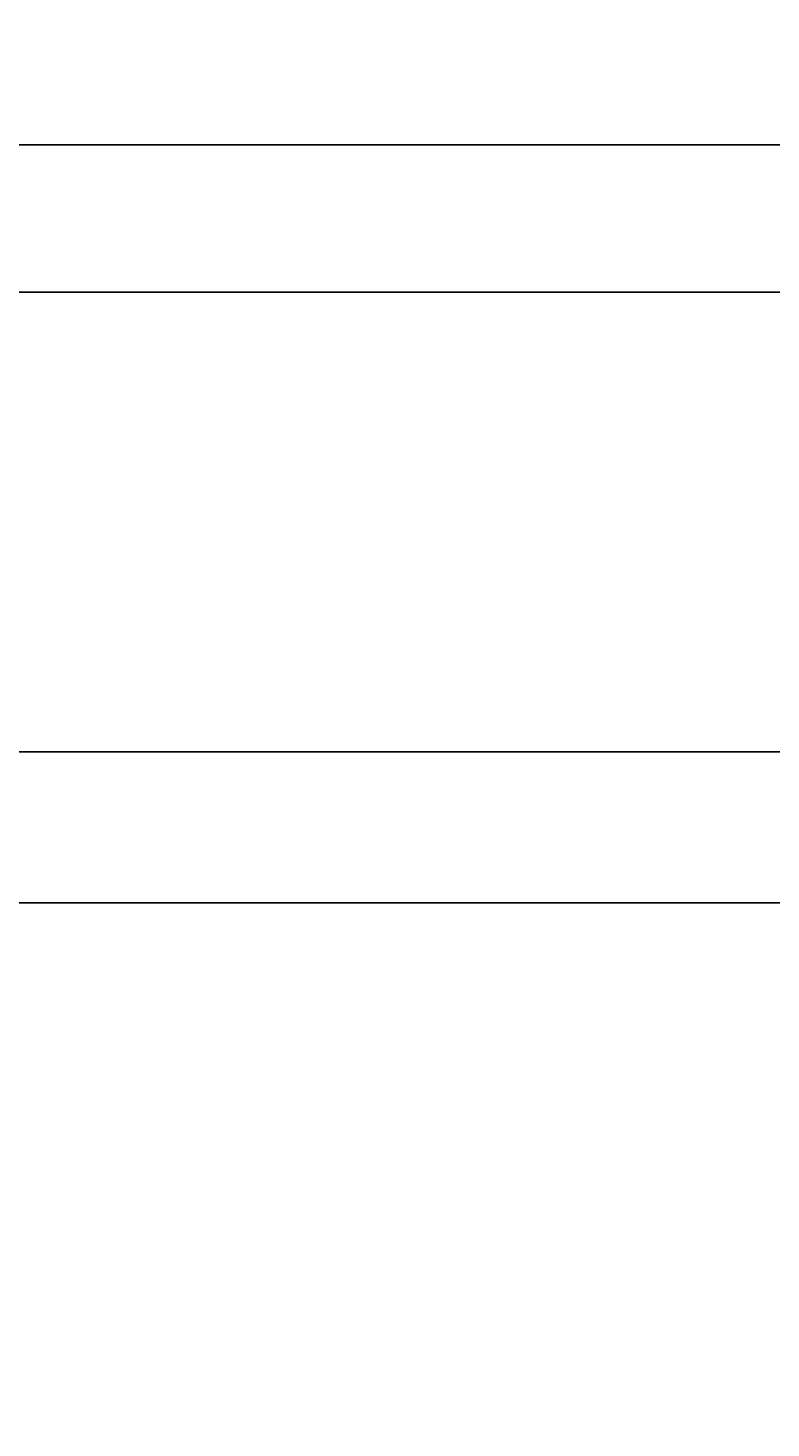
# Model space of a CAD drawing. Units: inches. Extents: x 35362 to 73946, y 43607 to 67532.
# Tile 73 of 134: x 49302 to 49711, y 46919 to 47689. Entities that reach past the tile are written whole.
import ezdxf

# ---------------------------------------------------------------- set-up
doc = ezdxf.new("R2010")
doc.units = ezdxf.units.IN
doc.header["$MEASUREMENT"] = 0
doc.layers.add('A-ANNO-DIMS', color=2, linetype='Continuous', lineweight=18)
doc.styles.get("Standard").update_dxf_attribs({"font": 'arial.ttf'})
doc.dimstyles.get("Standard").update_dxf_attribs({"dimtxt": 0.18, "dimasz": 0.18, "dimexe": 0.18, "dimexo": 0.0625, "dimgap": 0.09, "dimtad": 0, "dimtih": 1, "dimtoh": 1, "dimdec": 4, "dimzin": 0, "dimdsep": 46, "dimtxsty": 'Standard', "dimcen": 0.09, "dimadec": 0, "dimazin": 0, "dimtfac": 1, "dimtdec": 4, "dimtofl": 0, "dimtmove": 0, "dimatfit": 3, "dimfxl": 1, "dimtolj": 1, "dimtzin": 0, "dimarcsym": 0})

# ---------------------------------------------------------------- blocks, each defined once
blk = doc.blocks.new('*D11')
at = {"layer": 'A-ANNO-DIMS', "color": 0, "lineweight": -2, "transparency": 16777216}
for p, q in [((47978.66, 56028.77), (47978.66, 43606.68)), ((53109.76, 56028.77), (53109.76, 43606.68)), ((47978.84, 43606.86), (50543.87, 43606.86)), ((53109.58, 43606.86), (50544.55, 43606.86))]:
    blk.add_line(p, q, dxfattribs=at)
at = {"layer": 'A-ANNO-DIMS', "color": 0, "transparency": 16777216}
for points in [[(47978.84, 43606.89), (47978.84, 43606.83), (47978.66, 43606.86)], [(53109.58, 43606.89), (53109.58, 43606.83), (53109.76, 43606.86)]]:
    blk.add_solid(points, dxfattribs=at)
at = {"layer": 'Defpoints', "color": 0, "transparency": 16777216}
for p in [(47978.66, 56028.84), (53109.76, 56028.84), (53109.76, 43606.86)]:
    blk.add_point(p, dxfattribs=at)
at = {"layer": 'A-ANNO-DIMS', "color": 0, "transparency": 16777216, "insert": (50544.21, 43606.86), "char_height": 0.18, "attachment_point": 5}
blk.add_mtext('\\A1;5131', dxfattribs=at)
blk = doc.blocks.new('*D13')
at = {"layer": 'A-ANNO-DIMS', "color": 0, "lineweight": -2, "transparency": 16777216}
for p, q in [((48373.49, 51694.02), (48373.49, 43606.68)), ((51029.04, 51694.02), (51029.04, 43606.68)), ((48373.67, 43606.86), (49700.8, 43606.86)), ((51028.86, 43606.86), (49701.73, 43606.86))]:
    blk.add_line(p, q, dxfattribs=at)
at = {"layer": 'A-ANNO-DIMS', "color": 0, "transparency": 16777216}
for points in [[(48373.67, 43606.89), (48373.67, 43606.83), (48373.49, 43606.86)], [(51028.86, 43606.89), (51028.86, 43606.83), (51029.04, 43606.86)]]:
    blk.add_solid(points, dxfattribs=at)
at = {"layer": 'Defpoints', "color": 0, "transparency": 16777216}
for p in [(48373.49, 51694.09), (51029.04, 51694.09), (51029.04, 43606.86)]:
    blk.add_point(p, dxfattribs=at)
at = {"layer": 'A-ANNO-DIMS', "color": 0, "transparency": 16777216, "insert": (49701.27, 43606.86), "char_height": 0.18, "attachment_point": 5}
blk.add_mtext('\\A1;2655.6', dxfattribs=at)
blk = doc.blocks.new('*D43')
at = {"layer": 'A-ANNO-DIMS', "color": 0, "lineweight": -2, "transparency": 16777216}
for p, q in [((62004.67, 47625.18), (35361.77, 47625.18)), ((35361.95, 47625), (35361.95, 47416.9)), ((35361.95, 47208.43), (35361.95, 47416.53)), ((62004.67, 47208.25), (35361.77, 47208.25))]:
    blk.add_line(p, q, dxfattribs=at)
at = {"layer": 'A-ANNO-DIMS', "color": 0, "transparency": 16777216}
for points in [[(35361.92, 47625), (35361.98, 47625), (35361.95, 47625.18)], [(35361.92, 47208.43), (35361.98, 47208.43), (35361.95, 47208.25)]]:
    blk.add_solid(points, dxfattribs=at)
at = {"layer": 'Defpoints', "color": 0, "transparency": 16777216}
for p in [(62004.73, 47625.18), (35361.95, 47208.25), (62004.73, 47208.25)]:
    blk.add_point(p, dxfattribs=at)
at = {"layer": 'A-ANNO-DIMS', "color": 0, "transparency": 16777216, "insert": (35361.95, 47416.72), "char_height": 0.18, "attachment_point": 5}
blk.add_mtext('\\A1;416.9', dxfattribs=at)
blk = doc.blocks.new('*D67')
at = {"layer": 'A-ANNO-DIMS', "color": 0, "lineweight": -2, "transparency": 16777216}
for p, q in [((56873.54, 53351.53), (35361.77, 53351.53)), ((35361.95, 53351.35), (35361.95, 49400.89)), ((35361.95, 45450.07), (35361.95, 49400.53)), ((53793.58, 45449.89), (35361.77, 45449.89))]:
    blk.add_line(p, q, dxfattribs=at)
at = {"layer": 'A-ANNO-DIMS', "color": 0, "transparency": 16777216}
for points in [[(35361.92, 53351.35), (35361.98, 53351.35), (35361.95, 53351.53)], [(35361.92, 45450.07), (35361.98, 45450.07), (35361.95, 45449.89)]]:
    blk.add_solid(points, dxfattribs=at)
at = {"layer": 'Defpoints', "color": 0, "transparency": 16777216}
for p in [(35361.95, 53351.53), (56873.6, 53351.53), (53793.64, 45449.89)]:
    blk.add_point(p, dxfattribs=at)
at = {"layer": 'A-ANNO-DIMS', "color": 0, "transparency": 16777216, "insert": (35361.95, 49400.71), "char_height": 0.18, "attachment_point": 5}
blk.add_mtext('\\A1;7901.6', dxfattribs=at)
blk = doc.blocks.new('*D87')
at = {"layer": 'A-ANNO-DIMS', "color": 0, "lineweight": -2, "transparency": 16777216}
for p, q in [((52362.49, 48318.27), (35361.77, 48318.27)), ((35361.95, 48318.09), (35361.95, 47931.38)), ((35361.95, 47544.31), (35361.95, 47931.02)), ((52362.49, 47544.13), (35361.77, 47544.13))]:
    blk.add_line(p, q, dxfattribs=at)
at = {"layer": 'A-ANNO-DIMS', "color": 0, "transparency": 16777216}
for points in [[(35361.92, 48318.09), (35361.98, 48318.09), (35361.95, 48318.27)], [(35361.92, 47544.31), (35361.98, 47544.31), (35361.95, 47544.13)]]:
    blk.add_solid(points, dxfattribs=at)
at = {"layer": 'Defpoints', "color": 0, "transparency": 16777216}
for p in [(35361.95, 48318.27), (52362.56, 48318.27), (52362.56, 47544.13)]:
    blk.add_point(p, dxfattribs=at)
at = {"layer": 'A-ANNO-DIMS', "color": 0, "transparency": 16777216, "insert": (35361.95, 47931.2), "char_height": 0.18, "attachment_point": 5}
blk.add_mtext('\\A1;774.1', dxfattribs=at)
blk = doc.blocks.new('*D90')
at = {"layer": 'A-ANNO-DIMS', "color": 0, "lineweight": -2, "transparency": 16777216}
for p, q in [((53707.72, 47291.29), (35361.77, 47291.29)), ((35361.95, 47291.11), (35361.95, 46710.26)), ((35361.95, 46129.06), (35361.95, 46709.9)), ((53793.58, 46128.88), (35361.77, 46128.88))]:
    blk.add_line(p, q, dxfattribs=at)
at = {"layer": 'A-ANNO-DIMS', "color": 0, "transparency": 16777216}
for points in [[(35361.92, 47291.11), (35361.98, 47291.11), (35361.95, 47291.29)], [(35361.92, 46129.06), (35361.98, 46129.06), (35361.95, 46128.88)]]:
    blk.add_solid(points, dxfattribs=at)
at = {"layer": 'Defpoints', "color": 0, "transparency": 16777216}
for p in [(53707.78, 47291.29), (35361.95, 46128.88), (53793.64, 46128.88)]:
    blk.add_point(p, dxfattribs=at)
at = {"layer": 'A-ANNO-DIMS', "color": 0, "transparency": 16777216, "insert": (35361.95, 46710.08), "char_height": 0.18, "attachment_point": 5}
blk.add_mtext('\\A1;1162.4', dxfattribs=at)

msp = doc.modelspace()

# ---------------------------------------------------------------- dimensions: what is measured, and where the dimension line sits
at = {"layer": 'A-ANNO-DIMS'}
for base, p1, p2, override, picture, middle in [((53109.76, 43606.859), (47978.665, 56028.836), (53109.76, 56028.836), {"dimdec": 0, "dimlfac": 1, "dimrnd": 0, "dimzin": 0, "dimdsep": 46, "dimlunit": 2}, '*D11', (50544.212, 43606.859)), ((51029.043, 43606.859), (48373.492, 51694.087), (51029.043, 51694.087), {"dimdec": 1, "dimlfac": 1, "dimrnd": 0, "dimzin": 0, "dimdsep": 46, "dimlunit": 2}, '*D13', (49701.267, 43606.859))]:
    dim = msp.add_linear_dim(base=base, p1=p1, p2=p2, dimstyle='Standard', override=override, dxfattribs=at)
    dim.commit()
    dim.dimension.update_dxf_attribs({"geometry": picture, "text_midpoint": middle})
for base, p1, p2, picture, middle in [((35361.949, 53351.529), (53793.638, 45449.894), (56873.602, 53351.529), '*D67', (35361.949, 49400.712)), ((35361.949, 48318.269), (52362.557, 47544.134), (52362.557, 48318.269), '*D87', (35361.949, 47931.201)), ((35361.949, 47208.25), (62004.728, 47625.181), (62004.728, 47208.25), '*D43', (35361.949, 47416.715)), ((35361.949, 46128.878), (53707.781, 47291.285), (53793.638, 46128.878), '*D90', (35361.949, 46710.081))]:
    dim = msp.add_linear_dim(base=base, p1=p1, p2=p2, angle=90, dimstyle='Standard', override={"dimdec": 1, "dimlfac": 1, "dimrnd": 0, "dimzin": 0, "dimdsep": 46, "dimlunit": 2}, dxfattribs=at)
    dim.commit()
    dim.dimension.update_dxf_attribs({"geometry": picture, "text_midpoint": middle})

doc.saveas('drawing.dxf')
